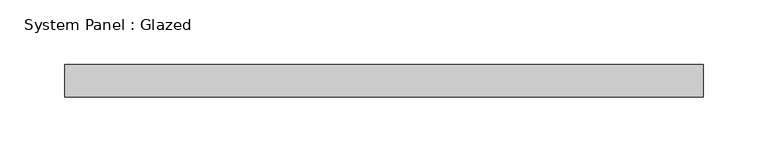
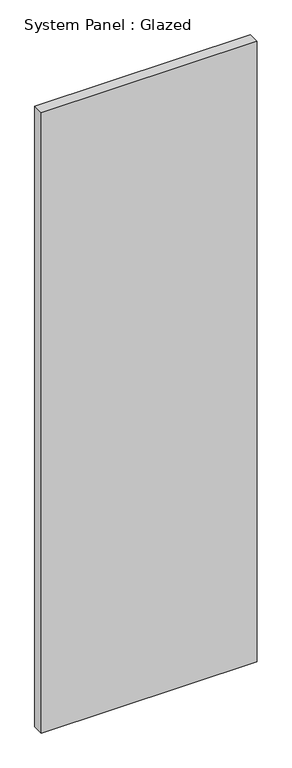
"""IFC4 building model written with IfcOpenShell, lengths in millimetres: plate geometry, System Panel : Glazed."""

from ifc_helpers import new_model, si_unit, origin, origin_with_axes, place, context, project, spatial, polyline, outline, extrude, source, transform, mapped, element, save


def system_panel_glazed_a9878b85(model_context):
    return source(origin(), model_context, "Body", "SweptSolid", [
        extrude(outline(polyline([(247.65, 19.05), (-247.65, 19.05), (-247.65, 44.45), (247.65, 44.45), (247.65, 19.05)])), origin_with_axes(), (0.0, 0.0, 1.0), 1503.931829),
    ])


if __name__ == "__main__":
    model = new_model("IFC4")
    model_context = context("Model", 3, world=origin())
    ifc_project = project(units=[si_unit("LENGTHUNIT", "METRE", prefix="MILLI")], contexts=[model_context])
    site = spatial("IfcSite", under=ifc_project)
    building = spatial("IfcBuilding", under=site)
    placement = place(None, origin())
    system_panel_glazed_shape = system_panel_glazed_a9878b85(model_context)
    element("IfcPlate", 1, ObjectType="System Panel : Glazed", at=placement, inside=building, context=model_context, shape_type="MappedRepresentation", body=[
        mapped(system_panel_glazed_shape, transform((0.0, 0.0, 0.0), x_axis=(1.0, 0.0, 0.0), y_axis=(0.0, 1.0, 0.0), z_axis=(0.0, 0.0, 1.0))),
    ])
    save(model, "model.ifc")

# Revit data of these elements
# Type "System Panel : Glazed"
#   Construction Type Id = "GSP4R"
#   Analytic Construction = "1/8 in Pilkington single glazing"
#   Visual Light Transmittance = 0.9
#   Solar Heat Gain Coefficient = 0.86
#   Heat Transfer Coefficient (U) = 1.18115 BTU/(h·ft²·°F)
#   Define Thermal Properties by = 1
# Element 1 (IfcPlate, "System Panel : Glazed")
#   Materials on its faces: "Glass"
# Materials
#   "Glass": class "Glass", colour RGB 0 128 192, transparency 0.75, Description = "Soda Lime Glass", Cost = 0
